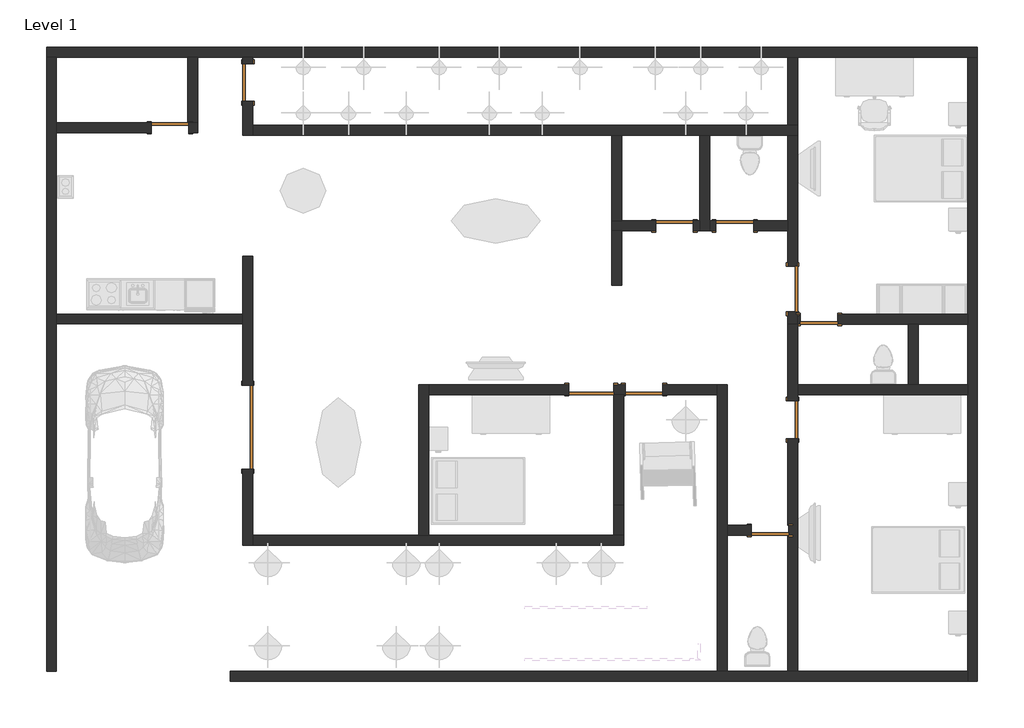
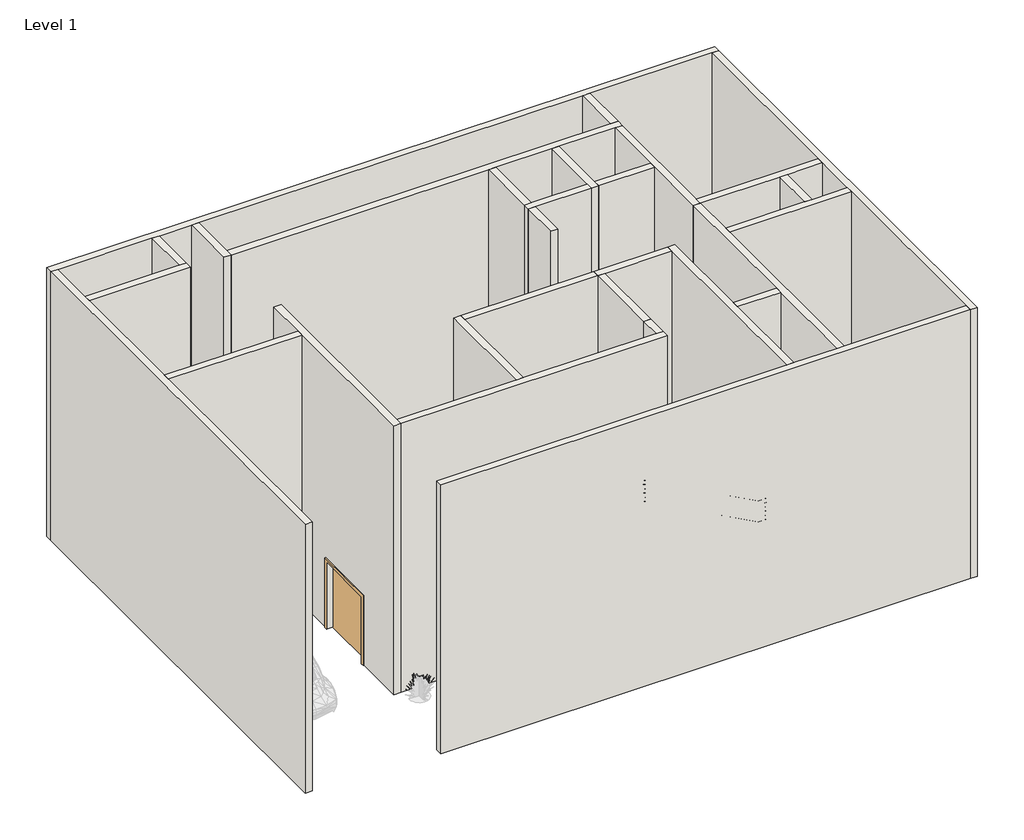
# One storey, part 1 of 4: 29 walls, 11 doors.
"""IFC4 building model written with IfcOpenShell, lengths in millimetres."""

from ifc_helpers import new_model, si_unit, frame, origin, origin_with_axes, place, context, project, spatial, polyline, outline, extrude, faceted_brep, transform, mapped, element, save
from components import m_door_double_flush_panel_double_acting_1700_x_2000mm_0a6d9c7f, m_single_flush_0762_x_2032mm_0c256fab, m_single_flush_0762_x_2032mm_7341a4fb, m_single_flush_0915_x_2032mm_26613924, m_single_flush_0915_x_2134mm_6a9e8738

model = new_model("IFC4")

# Units and contexts
model_context = context("Model", 3, world=origin())
ifc_project = project(units=[si_unit("LENGTHUNIT", "METRE", prefix="MILLI")], contexts=[model_context])

# Site, building, storey
site = spatial("IfcSite", under=ifc_project)
building = spatial("IfcBuilding", under=site)
storey = spatial("IfcBuildingStorey", under=building, Name="Level 1", Elevation=0.0)

# Doors
placement = place(None, origin())
m_door_double_flush_panel_double_acting_1700_x_2000mm_shape = m_door_double_flush_panel_double_acting_1700_x_2000mm_0a6d9c7f(model_context)
element("IfcDoor", 1, ObjectType="M_Door-Double-Flush_Panel-Double-Acting : 1700 x 2000mm", at=placement, inside=storey, context=model_context, shape_type="MappedRepresentation", body=[
    mapped(m_door_double_flush_panel_double_acting_1700_x_2000mm_shape, transform((-5650.4268643, 2289.4971112, 0.0), x_axis=(0.0, -1.0, 0.0), y_axis=(1.0, 0.0, 0.0), z_axis=(0.0, 0.0, 1.0))),
])
m_single_flush_0762_x_2032mm_shape = m_single_flush_0762_x_2032mm_0c256fab(model_context)
element("IfcDoor", 2, ObjectType="M_Single-Flush : 0762 x 2032mm", at=placement, inside=storey, context=model_context, shape_type="MappedRepresentation", body=[
    mapped(m_single_flush_0762_x_2032mm_shape, transform((-7222.0268643, 8333.0971112, 0.0), x_axis=(1.0, 0.0, 0.0), y_axis=(0.0, 1.0, 0.0), z_axis=(0.0, 0.0, 1.0))),
])
element("IfcDoor", 3, ObjectType="M_Single-Flush : 0762 x 2032mm", at=placement, inside=storey, context=model_context, shape_type="MappedRepresentation", body=[
    mapped(m_single_flush_0762_x_2032mm_shape, transform((-5648.8268643, 9249.0971112, 0.0), x_axis=(0.0, 1.0, 0.0), y_axis=(-1.0, 0.0, 0.0), z_axis=(0.0, 0.0, 1.0))),
])
element("IfcDoor", 4, ObjectType="M_Single-Flush : 0762 x 2032mm", at=placement, inside=storey, context=model_context, shape_type="MappedRepresentation", body=[
    mapped(m_single_flush_0762_x_2032mm_shape, transform((2963.3731357, 6351.8971112, 0.0), x_axis=(1.0, 0.0, 0.0), y_axis=(0.0, 1.0, 0.0), z_axis=(0.0, 0.0, 1.0))),
])
element("IfcDoor", 5, ObjectType="M_Single-Flush : 0762 x 2032mm", at=placement, inside=storey, context=model_context, shape_type="MappedRepresentation", body=[
    mapped(m_single_flush_0762_x_2032mm_shape, transform((5882.7731357, 4465.8971112, 0.0), x_axis=(-1.0, 0.0, 0.0), y_axis=(0.0, -1.0, 0.0), z_axis=(0.0, 0.0, 1.0))),
])
element("IfcDoor", 6, ObjectType="M_Single-Flush : 0762 x 2032mm", at=placement, inside=storey, context=model_context, shape_type="MappedRepresentation", body=[
    mapped(m_single_flush_0762_x_2032mm_shape, transform((2350.5731357, 3046.6971112, 0.0), x_axis=(-1.0, 0.0, 0.0), y_axis=(0.0, -1.0, 0.0), z_axis=(0.0, 0.0, 1.0))),
])
m_single_flush_0762_x_2032mm_2_shape = m_single_flush_0762_x_2032mm_7341a4fb(model_context)
element("IfcDoor", 7, ObjectType="M_Single-Flush : 0762 x 2032mm", at=placement, inside=storey, context=model_context, shape_type="MappedRepresentation", body=[
    mapped(m_single_flush_0762_x_2032mm_2_shape, transform((4182.5731357, 6351.8971112, 0.0), x_axis=(-1.0, 0.0, 0.0), y_axis=(0.0, -1.0, 0.0), z_axis=(0.0, 0.0, 1.0))),
])
element("IfcDoor", 8, ObjectType="M_Single-Flush : 0762 x 2032mm", at=placement, inside=storey, context=model_context, shape_type="MappedRepresentation", body=[
    mapped(m_single_flush_0762_x_2032mm_2_shape, transform((5349.3731357, 2437.0971112, 0.0), x_axis=(0.0, 1.0, 0.0), y_axis=(-1.0, 0.0, 0.0), z_axis=(0.0, 0.0, 1.0))),
])
element("IfcDoor", 9, ObjectType="M_Single-Flush : 0762 x 2032mm", at=placement, inside=storey, context=model_context, shape_type="MappedRepresentation", body=[
    mapped(m_single_flush_0762_x_2032mm_2_shape, transform((4892.1731357, 206.6971112, 0.0), x_axis=(1.0, 0.0, 0.0), y_axis=(0.0, 1.0, 0.0), z_axis=(0.0, 0.0, 1.0))),
])
m_single_flush_0915_x_2032mm_shape = m_single_flush_0915_x_2032mm_26613924(model_context)
element("IfcDoor", 10, ObjectType="M_Single-Flush : 0915 x 2032mm", at=placement, inside=storey, context=model_context, shape_type="MappedRepresentation", body=[
    mapped(m_single_flush_0915_x_2032mm_shape, transform((1283.7731357, 3046.6971112, 0.0), x_axis=(1.0, 0.0, 0.0), y_axis=(0.0, 1.0, 0.0), z_axis=(0.0, 0.0, 1.0))),
])
m_single_flush_0915_x_2134mm_shape = m_single_flush_0915_x_2134mm_6a9e8738(model_context)
element("IfcDoor", 11, ObjectType="M_Single-Flush : 0915 x 2134mm", at=placement, inside=storey, context=model_context, shape_type="MappedRepresentation", body=[
    mapped(m_single_flush_0915_x_2134mm_shape, transform((5349.3731357, 5075.4971112, 0.0), x_axis=(0.0, -1.0, 0.0), y_axis=(1.0, 0.0, 0.0), z_axis=(0.0, 0.0, 1.0))),
])

# Walls
element("IfcWall", 12, ObjectType="Generic - 200mm", at=placement, inside=storey, context=model_context, shape_type="Brep", body=[
    faceted_brep([(-9712.8268643, 9758.6971112, 0.0), (-9512.8268643, 9758.6971112, 0.0), (-6864.8268643, 9758.6971112, 0.0), (-6664.8268643, 9758.6971112, 0.0), (-5748.8268643, 9758.6971112, 0.0), (-5548.8268643, 9758.6971112, 0.0), (5249.3731357, 9758.6971112, 0.0), (5449.3731357, 9758.6971112, 0.0), (8879.9731357, 9758.6971112, 0.0), (9079.9731357, 9758.6971112, 0.0), (9079.9731357, 9758.6971112, 8000.0), (8879.9731357, 9758.6971112, 8000.0), (5449.3731357, 9758.6971112, 8000.0), (5249.3731357, 9758.6971112, 8000.0), (-5548.8268643, 9758.6971112, 8000.0), (-5748.8268643, 9758.6971112, 8000.0), (-6664.8268643, 9758.6971112, 8000.0), (-6864.8268643, 9758.6971112, 8000.0), (-9512.8268643, 9758.6971112, 8000.0), (-9712.8268643, 9758.6971112, 8000.0), (-9712.8268643, 9958.6971112, 0.0), (-9712.8268643, 9958.6971112, 8000.0), (9079.9731357, 9958.6971112, 8000.0), (9079.9731357, 9958.6971112, 0.0)], [[[0, 1, 2, 3, 4, 5, 6, 7, 8, 9, 10, 11, 12, 13, 14, 15, 16, 17, 18, 19]], [[20, 21, 22, 23]], [[9, 8, 7, 6, 5, 4, 3, 2, 1, 0, 20, 23]], [[19, 18, 17, 16, 15, 14, 13, 12, 11, 10, 22, 21]], [[10, 9, 23, 22]], [[0, 19, 21, 20]]]),
])
element("IfcWall", 13, ObjectType="Generic - 200mm", at=placement, inside=storey, context=model_context, shape_type="Brep", body=[
    faceted_brep([(8879.9731357, 9758.6971112, 0.0), (8879.9731357, 4565.8971112, 0.0), (8879.9731357, 4365.8971112, 0.0), (8879.9731357, 3146.6971112, 0.0), (8879.9731357, 2946.6971112, 0.0), (8879.9731357, -2638.1028888, 0.0), (8879.9731357, -2838.1028888, 0.0), (8879.9731357, -2838.1028888, 8000.0), (8879.9731357, -2638.1028888, 8000.0), (8879.9731357, 2946.6971112, 8000.0), (8879.9731357, 3146.6971112, 8000.0), (8879.9731357, 4365.8971112, 8000.0), (8879.9731357, 4565.8971112, 8000.0), (8879.9731357, 9758.6971112, 8000.0), (9079.9731357, 9758.6971112, 0.0), (9079.9731357, 9758.6971112, 8000.0), (9079.9731357, -2838.1028888, 8000.0), (9079.9731357, -2838.1028888, 0.0)], [[[0, 1, 2, 3, 4, 5, 6, 7, 8, 9, 10, 11, 12, 13]], [[14, 15, 16, 17]], [[6, 5, 4, 3, 2, 1, 0, 14, 17]], [[13, 12, 11, 10, 9, 8, 7, 16, 15]], [[0, 13, 15, 14]], [[7, 6, 17, 16]]]),
])
element("IfcWall", 14, ObjectType="Generic - 200mm", at=placement, inside=storey, context=model_context, shape_type="Brep", body=[
    faceted_brep([(-9512.8268643, -2638.1028888, 0.0), (-9512.8268643, 4372.2971112, 0.0), (-9512.8268643, 4572.2971112, 0.0), (-9512.8268643, 8233.0971112, 0.0), (-9512.8268643, 8433.0971112, 0.0), (-9512.8268643, 9758.6971112, 0.0), (-9512.8268643, 9758.6971112, 8000.0), (-9512.8268643, 8433.0971112, 8000.0), (-9512.8268643, 8233.0971112, 8000.0), (-9512.8268643, 4572.2971112, 8000.0), (-9512.8268643, 4372.2971112, 8000.0), (-9512.8268643, -2638.1028888, 8000.0), (-9712.8268643, -2638.1028888, 0.0), (-9712.8268643, -2638.1028888, 8000.0), (-9712.8268643, 9758.6971112, 8000.0), (-9712.8268643, 9758.6971112, 0.0)], [[[0, 1, 2, 3, 4, 5, 6, 7, 8, 9, 10, 11]], [[12, 13, 14, 15]], [[5, 4, 3, 2, 1, 0, 12, 15]], [[11, 10, 9, 8, 7, 6, 14, 13]], [[0, 11, 13, 12]], [[6, 5, 15, 14]]]),
])
element("IfcWall", 15, ObjectType="Generic - 200mm", at=placement, inside=storey, context=model_context, shape_type="Brep", body=[
    faceted_brep([(-6841.0268643, 8233.0971112, 2032.0), (-6841.0268643, 8233.0971112, 0.0), (-6664.8268643, 8233.0971112, 0.0), (-6664.8268643, 8233.0971112, 8000.0), (-9512.8268643, 8233.0971112, 8000.0), (-9512.8268643, 8233.0971112, 0.0), (-7603.0268643, 8233.0971112, 0.0), (-7603.0268643, 8233.0971112, 2032.0), (-6664.8268643, 8433.0971112, 0.0), (-6841.0268643, 8433.0971112, 0.0), (-6841.0268643, 8433.0971112, 2032.0), (-7603.0268643, 8433.0971112, 2032.0), (-7603.0268643, 8433.0971112, 0.0), (-9512.8268643, 8433.0971112, 0.0), (-9512.8268643, 8433.0971112, 8000.0), (-6864.8268643, 8433.0971112, 8000.0), (-6664.8268643, 8433.0971112, 8000.0)], [[[0, 1, 2, 3, 4, 5, 6, 7]], [[8, 9, 10, 11, 12, 13, 14, 15, 16]], [[6, 5, 13, 12]], [[2, 1, 9, 8]], [[4, 3, 16, 15, 14]], [[5, 4, 14, 13]], [[3, 2, 8, 16]], [[10, 9, 1, 0]], [[11, 10, 0, 7]], [[12, 11, 7, 6]]]),
])
element("IfcWall", 16, ObjectType="Generic - 200mm", at=placement, inside=storey, context=model_context, shape_type="SweptSolid", body=[
    extrude(outline(polyline([(-6664.8268643, 9758.6971112), (-6664.8268643, 8433.0971112), (-6864.8268643, 8433.0971112), (-6864.8268643, 9758.6971112), (-6664.8268643, 9758.6971112)])), origin_with_axes(), (0.0, 0.0, 1.0), 8000.0),
])
element("IfcWall", 17, ObjectType="Generic - 200mm", at=placement, inside=storey, context=model_context, shape_type="SweptSolid", body=[
    extrude(outline(polyline([(-5750.4268643, 4372.2971112), (-9512.8268643, 4372.2971112), (-9512.8268643, 4572.2971112), (-5750.4268643, 4572.2971112), (-5750.4268643, 4372.2971112)])), origin_with_axes(), (0.0, 0.0, 1.0), 8000.0),
])
element("IfcWall", 18, ObjectType="Generic - 200mm", at=placement, inside=storey, context=model_context, shape_type="Brep", body=[
    faceted_brep([(-5550.4268643, 5743.8971112, 0.0), (-5550.4268643, 5743.8971112, 8000.0), (-5550.4268643, 106.6971112, 8000.0), (-5550.4268643, -93.3028888, 8000.0), (-5550.4268643, -93.3028888, 0.0), (-5550.4268643, 106.6971112, 0.0), (-5550.4268643, 1439.4971112, 0.0), (-5550.4268643, 1439.4971112, 2000.0), (-5550.4268643, 3139.4971112, 2000.0), (-5550.4268643, 3139.4971112, 0.0), (-5750.4268643, 5743.8971112, 8000.0), (-5750.4268643, 5743.8971112, 0.0), (-5750.4268643, 4572.2971112, 0.0), (-5750.4268643, 4372.2971112, 0.0), (-5750.4268643, 3139.4971112, 0.0), (-5750.4268643, 3139.4971112, 2000.0), (-5750.4268643, 1439.4971112, 2000.0), (-5750.4268643, 1439.4971112, 0.0), (-5750.4268643, -93.3028888, 0.0), (-5750.4268643, -93.3028888, 8000.0), (-5750.4268643, 4372.2971112, 8000.0), (-5750.4268643, 4572.2971112, 8000.0)], [[[0, 1, 2, 3, 4, 5, 6, 7, 8, 9]], [[10, 11, 12, 13, 14, 15, 16, 17, 18, 19, 20, 21]], [[11, 0, 9, 14, 13, 12]], [[4, 18, 17, 6, 5]], [[1, 0, 11, 10]], [[3, 2, 1, 10, 21, 20, 19]], [[16, 7, 6, 17]], [[7, 16, 15, 8]], [[8, 15, 14, 9]], [[4, 3, 19, 18]]]),
])
element("IfcWall", 19, ObjectType="Generic - 200mm", at=placement, inside=storey, context=model_context, shape_type="Brep", body=[
    faceted_brep([(-5748.8268643, 9758.6971112, 0.0), (-5748.8268643, 9630.0971112, 0.0), (-5748.8268643, 9630.0971112, 2032.0), (-5748.8268643, 8868.0971112, 2032.0), (-5748.8268643, 8868.0971112, 0.0), (-5748.8268643, 8180.6971112, 0.0), (-5748.8268643, 8180.6971112, 8000.0), (-5748.8268643, 9758.6971112, 8000.0), (-5548.8268643, 9630.0971112, 2032.0), (-5548.8268643, 9630.0971112, 0.0), (-5548.8268643, 9758.6971112, 0.0), (-5548.8268643, 9758.6971112, 8000.0), (-5548.8268643, 8380.6971112, 8000.0), (-5548.8268643, 8180.6971112, 8000.0), (-5548.8268643, 8180.6971112, 0.0), (-5548.8268643, 8380.6971112, 0.0), (-5548.8268643, 8868.0971112, 0.0), (-5548.8268643, 8868.0971112, 2032.0)], [[[0, 1, 2, 3, 4, 5, 6, 7]], [[8, 9, 10, 11, 12, 13, 14, 15, 16, 17]], [[10, 9, 1, 0]], [[16, 15, 14, 5, 4]], [[6, 5, 14, 13]], [[7, 6, 13, 12, 11]], [[0, 7, 11, 10]], [[2, 1, 9, 8]], [[3, 2, 8, 17]], [[4, 3, 17, 16]]]),
])
element("IfcWall", 20, ObjectType="Generic - 200mm", at=placement, inside=storey, context=model_context, shape_type="Brep", body=[
    faceted_brep([(-5548.8268643, 8180.6971112, 0.0), (1694.9731357, 8180.6971112, 0.0), (1894.9731357, 8180.6971112, 0.0), (3472.9731357, 8180.6971112, 0.0), (3672.9731357, 8180.6971112, 0.0), (5249.3731357, 8180.6971112, 0.0), (5449.3731357, 8180.6971112, 0.0), (5449.3731357, 8180.6971112, 8000.0), (5249.3731357, 8180.6971112, 8000.0), (3672.9731357, 8180.6971112, 8000.0), (3472.9731357, 8180.6971112, 8000.0), (1894.9731357, 8180.6971112, 8000.0), (1694.9731357, 8180.6971112, 8000.0), (-5548.8268643, 8180.6971112, 8000.0), (-5548.8268643, 8380.6971112, 0.0), (-5548.8268643, 8380.6971112, 8000.0), (5249.3731357, 8380.6971112, 8000.0), (5449.3731357, 8380.6971112, 8000.0), (5449.3731357, 8380.6971112, 0.0), (5249.3731357, 8380.6971112, 0.0)], [[[0, 1, 2, 3, 4, 5, 6, 7, 8, 9, 10, 11, 12, 13]], [[14, 15, 16, 17, 18, 19]], [[6, 5, 4, 3, 2, 1, 0, 14, 19, 18]], [[13, 12, 11, 10, 9, 8, 7, 17, 16, 15]], [[0, 13, 15, 14]], [[7, 6, 18, 17]]]),
])
element("IfcWall", 21, ObjectType="Generic - 200mm", at=placement, inside=storey, context=model_context, shape_type="SweptSolid", body=[
    extrude(outline(polyline([(5449.3731357, 9758.6971112), (5449.3731357, 8380.6971112), (5249.3731357, 8380.6971112), (5249.3731357, 9758.6971112), (5449.3731357, 9758.6971112)])), origin_with_axes(), (0.0, 0.0, 1.0), 8000.0),
])
element("IfcWall", 22, ObjectType="Generic - 200mm", at=placement, inside=storey, context=model_context, shape_type="Brep", body=[
    faceted_brep([(5249.3731357, 4617.9971112, 2134.0), (5249.3731357, 4617.9971112, 0.0), (5249.3731357, 4365.8971112, 0.0), (5249.3731357, 4365.8971112, 8000.0), (5249.3731357, 6251.8971112, 8000.0), (5249.3731357, 6451.8971112, 8000.0), (5249.3731357, 8180.6971112, 8000.0), (5249.3731357, 8180.6971112, 0.0), (5249.3731357, 6451.8971112, 0.0), (5249.3731357, 6251.8971112, 0.0), (5249.3731357, 5532.9971112, 0.0), (5249.3731357, 5532.9971112, 2134.0), (5449.3731357, 4365.8971112, 0.0), (5449.3731357, 4565.8971112, 0.0), (5449.3731357, 4617.9971112, 0.0), (5449.3731357, 4617.9971112, 2134.0), (5449.3731357, 5532.9971112, 2134.0), (5449.3731357, 5532.9971112, 0.0), (5449.3731357, 8180.6971112, 0.0), (5449.3731357, 8180.6971112, 8000.0), (5449.3731357, 4565.8971112, 8000.0), (5449.3731357, 4365.8971112, 8000.0)], [[[0, 1, 2, 3, 4, 5, 6, 7, 8, 9, 10, 11]], [[12, 13, 14, 15, 16, 17, 18, 19, 20, 21]], [[2, 1, 14, 13, 12]], [[10, 9, 8, 7, 18, 17]], [[6, 5, 4, 3, 21, 20, 19]], [[7, 6, 19, 18]], [[3, 2, 12, 21]], [[15, 14, 1, 0]], [[16, 15, 0, 11]], [[17, 16, 11, 10]]]),
])
element("IfcWall", 23, ObjectType="Generic - 200mm", at=placement, inside=storey, context=model_context, shape_type="Brep", body=[
    faceted_brep([(5449.3731357, 4365.8971112, 0.0), (5501.7731357, 4365.8971112, 0.0), (5501.7731357, 4365.8971112, 2032.0), (6263.7731357, 4365.8971112, 2032.0), (6263.7731357, 4365.8971112, 0.0), (7684.5731357, 4365.8971112, 0.0), (7884.5731357, 4365.8971112, 0.0), (8879.9731357, 4365.8971112, 0.0), (8879.9731357, 4365.8971112, 8000.0), (7884.5731357, 4365.8971112, 8000.0), (7684.5731357, 4365.8971112, 8000.0), (5449.3731357, 4365.8971112, 8000.0), (5501.7731357, 4565.8971112, 2032.0), (5501.7731357, 4565.8971112, 0.0), (5449.3731357, 4565.8971112, 0.0), (5449.3731357, 4565.8971112, 8000.0), (8879.9731357, 4565.8971112, 8000.0), (8879.9731357, 4565.8971112, 0.0), (6263.7731357, 4565.8971112, 0.0), (6263.7731357, 4565.8971112, 2032.0)], [[[0, 1, 2, 3, 4, 5, 6, 7, 8, 9, 10, 11]], [[12, 13, 14, 15, 16, 17, 18, 19]], [[18, 17, 7, 6, 5, 4]], [[14, 13, 1, 0]], [[11, 10, 9, 8, 16, 15]], [[0, 11, 15, 14]], [[8, 7, 17, 16]], [[2, 1, 13, 12]], [[3, 2, 12, 19]], [[4, 3, 19, 18]]]),
])
element("IfcWall", 24, ObjectType="Generic - 200mm", at=placement, inside=storey, context=model_context, shape_type="Brep", body=[
    faceted_brep([(3472.9731357, 8180.6971112, 0.0), (3472.9731357, 6451.8971112, 0.0), (3472.9731357, 6251.8971112, 0.0), (3472.9731357, 6251.8971112, 8000.0), (3472.9731357, 6451.8971112, 8000.0), (3472.9731357, 8180.6971112, 8000.0), (3672.9731357, 8180.6971112, 0.0), (3672.9731357, 8180.6971112, 8000.0), (3672.9731357, 6451.8971112, 8000.0), (3672.9731357, 6251.8971112, 8000.0), (3672.9731357, 6251.8971112, 0.0), (3672.9731357, 6451.8971112, 0.0)], [[[0, 1, 2, 3, 4, 5]], [[6, 7, 8, 9, 10, 11]], [[2, 1, 0, 6, 11, 10]], [[5, 4, 3, 9, 8, 7]], [[0, 5, 7, 6]], [[3, 2, 10, 9]]]),
])
element("IfcWall", 25, ObjectType="Generic - 200mm", at=placement, inside=storey, context=model_context, shape_type="SweptSolid", body=[
    extrude(outline(polyline([(0.0, 3672.9731357), (0.0, 3801.5731357), (2032.0, 3801.5731357), (2032.0, 4563.5731357), (0.0, 4563.5731357), (0.0, 5249.3731357), (8000.0, 5249.3731357), (8000.0, 3672.9731357), (0.0, 3672.9731357)])), frame((0.0, 6251.8971112, 0.0), z_axis=(0.0, 1.0, 0.0), x_axis=(0.0, 0.0, 1.0)), (0.0, 0.0, 1.0), 200.0),
])
element("IfcWall", 26, ObjectType="Generic - 200mm", at=placement, inside=storey, context=model_context, shape_type="Brep", body=[
    faceted_brep([(3472.9731357, 6451.8971112, 0.0), (3344.3731357, 6451.8971112, 0.0), (3344.3731357, 6451.8971112, 2032.0), (2582.3731357, 6451.8971112, 2032.0), (2582.3731357, 6451.8971112, 0.0), (1894.9731357, 6451.8971112, 0.0), (1694.9731357, 6451.8971112, 0.0), (1694.9731357, 6451.8971112, 8000.0), (1894.9731357, 6451.8971112, 8000.0), (3472.9731357, 6451.8971112, 8000.0), (3344.3731357, 6251.8971112, 2032.0), (3344.3731357, 6251.8971112, 0.0), (3472.9731357, 6251.8971112, 0.0), (3472.9731357, 6251.8971112, 8000.0), (1896.5731357, 6251.8971112, 8000.0), (1696.5731357, 6251.8971112, 8000.0), (1694.9731357, 6251.8971112, 8000.0), (1694.9731357, 6251.8971112, 0.0), (1696.5731357, 6251.8971112, 0.0), (1896.5731357, 6251.8971112, 0.0), (2582.3731357, 6251.8971112, 0.0), (2582.3731357, 6251.8971112, 2032.0)], [[[0, 1, 2, 3, 4, 5, 6, 7, 8, 9]], [[10, 11, 12, 13, 14, 15, 16, 17, 18, 19, 20, 21]], [[12, 11, 1, 0]], [[20, 19, 18, 17, 6, 5, 4]], [[9, 8, 7, 16, 15, 14, 13]], [[0, 9, 13, 12]], [[7, 6, 17, 16]], [[2, 1, 11, 10]], [[3, 2, 10, 21]], [[4, 3, 21, 20]]]),
])
element("IfcWall", 27, ObjectType="Generic - 200mm", at=placement, inside=storey, context=model_context, shape_type="SweptSolid", body=[
    extrude(outline(polyline([(1894.9731357, 8180.6971112), (1894.9731357, 6451.8971112), (1694.9731357, 6451.8971112), (1694.9731357, 8180.6971112), (1894.9731357, 8180.6971112)])), origin_with_axes(), (0.0, 0.0, 1.0), 8000.0),
])
element("IfcWall", 28, ObjectType="Generic - 200mm", at=placement, inside=storey, context=model_context, shape_type="Brep", body=[
    faceted_brep([(5249.3731357, -2638.1028888, 8000.0), (5249.3731357, 106.6971112, 8000.0), (5249.3731357, 306.6971112, 8000.0), (5249.3731357, 4365.8971112, 8000.0), (5249.3731357, 4365.8971112, 0.0), (5249.3731357, 2818.0971112, 0.0), (5249.3731357, 2818.0971112, 2032.0), (5249.3731357, 2056.0971112, 2032.0), (5249.3731357, 2056.0971112, 0.0), (5249.3731357, 306.6971112, 0.0), (5249.3731357, 306.6971112, 2032.0), (5249.3731357, 106.6971112, 2032.0), (5249.3731357, 106.6971112, 0.0), (5249.3731357, -2638.1028888, 0.0), (5449.3731357, 4365.8971112, 8000.0), (5449.3731357, 3146.6971112, 8000.0), (5449.3731357, 2946.6971112, 8000.0), (5449.3731357, -2638.1028888, 8000.0), (5449.3731357, -2638.1028888, 0.0), (5449.3731357, 2056.0971112, 0.0), (5449.3731357, 2056.0971112, 2032.0), (5449.3731357, 2818.0971112, 2032.0), (5449.3731357, 2818.0971112, 0.0), (5449.3731357, 2946.6971112, 0.0), (5449.3731357, 3146.6971112, 0.0), (5449.3731357, 4365.8971112, 0.0), (5273.1731357, 106.6971112, 0.0), (5273.1731357, 306.6971112, 0.0), (5273.1731357, 106.6971112, 2032.0), (5273.1731357, 306.6971112, 2032.0)], [[[0, 1, 2, 3, 4, 5, 6, 7, 8, 9, 10, 11, 12, 13]], [[14, 15, 16, 17, 18, 19, 20, 21, 22, 23, 24, 25]], [[4, 25, 24, 23, 22, 5]], [[8, 19, 18, 13, 12, 26, 27, 9]], [[3, 2, 1, 0, 17, 16, 15, 14]], [[4, 3, 14, 25]], [[6, 5, 22, 21]], [[7, 6, 21, 20]], [[8, 7, 20, 19]], [[28, 26, 12, 11]], [[27, 29, 10, 9]], [[26, 28, 29, 27]], [[29, 28, 11, 10]], [[0, 13, 18, 17]]]),
])
element("IfcWall", 29, ObjectType="Generic - 200mm", at=placement, inside=storey, context=model_context, shape_type="Brep", body=[
    faceted_brep([(5449.3731357, 2946.6971112, 0.0), (8879.9731357, 2946.6971112, 0.0), (8879.9731357, 2946.6971112, 8000.0), (5449.3731357, 2946.6971112, 8000.0), (5449.3731357, 3146.6971112, 0.0), (5449.3731357, 3146.6971112, 8000.0), (7684.5731357, 3146.6971112, 8000.0), (7884.5731357, 3146.6971112, 8000.0), (8879.9731357, 3146.6971112, 8000.0), (8879.9731357, 3146.6971112, 0.0), (7884.5731357, 3146.6971112, 0.0), (7684.5731357, 3146.6971112, 0.0)], [[[0, 1, 2, 3]], [[4, 5, 6, 7, 8, 9, 10, 11]], [[1, 0, 4, 11, 10, 9]], [[3, 2, 8, 7, 6, 5]], [[0, 3, 5, 4]], [[2, 1, 9, 8]]]),
])
element("IfcWall", 30, ObjectType="Generic - 200mm", at=placement, inside=storey, context=model_context, shape_type="SweptSolid", body=[
    extrude(outline(polyline([(7884.5731357, 4365.8971112), (7884.5731357, 3146.6971112), (7684.5731357, 3146.6971112), (7684.5731357, 4365.8971112), (7884.5731357, 4365.8971112)])), origin_with_axes(), (0.0, 0.0, 1.0), 8000.0),
])
element("IfcWall", 31, ObjectType="Generic - 200mm", at=placement, inside=storey, context=model_context, shape_type="SweptSolid", body=[
    extrude(outline(polyline([(1696.5731357, 5158.0971112), (1696.5731357, 6251.8971112), (1896.5731357, 6251.8971112), (1896.5731357, 5158.0971112), (1696.5731357, 5158.0971112)])), origin_with_axes(), (0.0, 0.0, 1.0), 8000.0),
])
element("IfcWall", 32, ObjectType="Generic - 200mm", at=placement, inside=storey, context=model_context, shape_type="Brep", body=[
    faceted_brep([(4026.9731357, -2638.1028888, 0.0), (4026.9731357, 106.6971112, 0.0), (4026.9731357, 306.6971112, 0.0), (4026.9731357, 3146.6971112, 0.0), (4026.9731357, 3146.6971112, 8000.0), (4026.9731357, 306.6971112, 8000.0), (4026.9731357, 106.6971112, 8000.0), (4026.9731357, -2638.1028888, 8000.0), (3826.9731357, -2638.1028888, 0.0), (3826.9731357, -2638.1028888, 8000.0), (3826.9731357, 2946.6971112, 8000.0), (3826.9731357, 3146.6971112, 8000.0), (3826.9731357, 3146.6971112, 0.0), (3826.9731357, 2946.6971112, 0.0)], [[[0, 1, 2, 3, 4, 5, 6, 7]], [[8, 9, 10, 11, 12, 13]], [[3, 2, 1, 0, 8, 13, 12]], [[7, 6, 5, 4, 11, 10, 9]], [[4, 3, 12, 11]], [[0, 7, 9, 8]]]),
])
element("IfcWall", 33, ObjectType="Generic - 200mm", at=placement, inside=storey, context=model_context, shape_type="SweptSolid", body=[
    extrude(outline(polyline([(8000.0, 5249.3731357), (8000.0, 4026.9731357), (0.0, 4026.9731357), (0.0, 4511.1731357), (2032.0, 4511.1731357), (2032.0, 5249.3731357), (8000.0, 5249.3731357)])), frame((0.0, 106.6971112, 0.0), z_axis=(0.0, 1.0, 0.0), x_axis=(0.0, 0.0, 1.0)), (0.0, 0.0, 1.0), 200.0),
])
element("IfcWall", 34, ObjectType="Generic - 200mm", at=placement, inside=storey, context=model_context, shape_type="Brep", body=[
    faceted_brep([(1969.5731357, 3146.6971112, 2032.0), (1969.5731357, 3146.6971112, 0.0), (1741.2731357, 3146.6971112, 0.0), (1741.2731357, 3146.6971112, 2032.0), (1740.9731357, 3146.6971112, 2032.0), (1740.9731357, 3146.6971112, 8000.0), (3826.9731357, 3146.6971112, 8000.0), (3826.9731357, 3146.6971112, 0.0), (2731.5731357, 3146.6971112, 0.0), (2731.5731357, 3146.6971112, 2032.0), (1741.2731357, 2946.6971112, 0.0), (1940.9731357, 2946.6971112, 0.0), (1969.5731357, 2946.6971112, 0.0), (1969.5731357, 2946.6971112, 2032.0), (2731.5731357, 2946.6971112, 2032.0), (2731.5731357, 2946.6971112, 0.0), (3826.9731357, 2946.6971112, 0.0), (3826.9731357, 2946.6971112, 8000.0), (1940.9731357, 2946.6971112, 8000.0), (1740.9731357, 2946.6971112, 8000.0), (1740.9731357, 2946.6971112, 2032.0), (1741.2731357, 2946.6971112, 2032.0)], [[[0, 1, 2, 3, 4, 5, 6, 7, 8, 9]], [[10, 11, 12, 13, 14, 15, 16, 17, 18, 19, 20, 21]], [[8, 7, 16, 15]], [[2, 1, 12, 11, 10]], [[6, 5, 19, 18, 17]], [[7, 6, 17, 16]], [[19, 5, 4, 20]], [[21, 3, 2, 10]], [[3, 21, 20, 4]], [[13, 12, 1, 0]], [[14, 13, 0, 9]], [[15, 14, 9, 8]]]),
])
element("IfcWall", 35, ObjectType="Generic - 200mm", at=placement, inside=storey, context=model_context, shape_type="Brep", body=[
    faceted_brep([(1740.9731357, 2946.6971112, 0.0), (1740.9731357, 708.2971112, 0.0), (1740.9731357, 708.2971112, 8000.0), (1740.9731357, 2946.6971112, 8000.0), (1740.9731357, 2946.6971112, 2032.0), (1940.9731357, 2946.6971112, 0.0), (1940.9731357, 2946.6971112, 8000.0), (1940.9731357, 708.2971112, 8000.0), (1940.9731357, 708.2971112, 0.0), (1741.2731357, 2946.6971112, 0.0)], [[[0, 1, 2, 3, 4]], [[5, 6, 7, 8]], [[1, 0, 9, 5, 8]], [[2, 1, 8, 7]], [[3, 2, 7, 6]], [[0, 4, 3, 6, 5, 9]]]),
])
element("IfcWall", 36, ObjectType="Generic - 200mm", at=placement, inside=storey, context=model_context, shape_type="Brep", body=[
    faceted_brep([(-5550.4268643, -93.3028888, 0.0), (1940.9731357, -93.3028888, 0.0), (1940.9731357, -93.3028888, 8000.0), (-5550.4268643, -93.3028888, 8000.0), (-5550.4268643, 106.6971112, 0.0), (-5550.4268643, 106.6971112, 8000.0), (-2194.4268643, 106.6971112, 8000.0), (-1994.4268643, 106.6971112, 8000.0), (1740.9731357, 106.6971112, 8000.0), (1940.9731357, 106.6971112, 8000.0), (1940.9731357, 106.6971112, 0.0), (1740.9731357, 106.6971112, 0.0), (-1994.4268643, 106.6971112, 0.0), (-2194.4268643, 106.6971112, 0.0)], [[[0, 1, 2, 3]], [[4, 5, 6, 7, 8, 9, 10, 11, 12, 13]], [[1, 0, 4, 13, 12, 11, 10]], [[3, 2, 9, 8, 7, 6, 5]], [[0, 3, 5, 4]], [[2, 1, 10, 9]]]),
])
element("IfcWall", 37, ObjectType="Generic - 200mm", at=placement, inside=storey, context=model_context, shape_type="Brep", body=[
    faceted_brep([(-1994.4268643, 106.6971112, 0.0), (-1994.4268643, 2946.6971112, 0.0), (-1994.4268643, 3146.6971112, 0.0), (-1994.4268643, 3146.6971112, 8000.0), (-1994.4268643, 2946.6971112, 8000.0), (-1994.4268643, 106.6971112, 8000.0), (-2194.4268643, 106.6971112, 0.0), (-2194.4268643, 106.6971112, 8000.0), (-2194.4268643, 3146.6971112, 8000.0), (-2194.4268643, 3146.6971112, 0.0)], [[[0, 1, 2, 3, 4, 5]], [[6, 7, 8, 9]], [[2, 1, 0, 6, 9]], [[5, 4, 3, 8, 7]], [[0, 5, 7, 6]], [[3, 2, 9, 8]]]),
])
element("IfcWall", 38, ObjectType="Generic - 200mm", at=placement, inside=storey, context=model_context, shape_type="SweptSolid", body=[
    extrude(outline(polyline([(8000.0, 1740.9731357), (8000.0, -1994.4268643), (0.0, -1994.4268643), (0.0, 826.2731357), (2032.0, 826.2731357), (2032.0, 1740.9731357), (8000.0, 1740.9731357)])), frame((0.0, 2946.6971112, 0.0), z_axis=(0.0, 1.0, 0.0), x_axis=(0.0, 0.0, 1.0)), (0.0, 0.0, 1.0), 200.0),
])
element("IfcWall", 39, ObjectType="Generic - 200mm", at=placement, inside=storey, context=model_context, shape_type="SweptSolid", body=[
    extrude(outline(polyline([(1940.9731357, 708.2971112), (1940.9731357, 106.6971112), (1740.9731357, 106.6971112), (1740.9731357, 708.2971112), (1940.9731357, 708.2971112)])), origin_with_axes(), (0.0, 0.0, 1.0), 8000.0),
])
element("IfcWall", 40, ObjectType="Generic - 200mm", at=placement, inside=storey, context=model_context, shape_type="Brep", body=[
    faceted_brep([(8879.9731357, -2638.1028888, 0.0), (5449.3731357, -2638.1028888, 0.0), (5249.3731357, -2638.1028888, 0.0), (4026.9731357, -2638.1028888, 0.0), (3826.9731357, -2638.1028888, 0.0), (-6007.6268643, -2638.1028888, 0.0), (-6007.6268643, -2638.1028888, 8000.0), (3826.9731357, -2638.1028888, 8000.0), (4026.9731357, -2638.1028888, 8000.0), (5249.3731357, -2638.1028888, 8000.0), (5449.3731357, -2638.1028888, 8000.0), (8879.9731357, -2638.1028888, 8000.0), (8879.9731357, -2838.1028888, 0.0), (8879.9731357, -2838.1028888, 8000.0), (-6007.6268643, -2838.1028888, 8000.0), (-6007.6268643, -2838.1028888, 0.0)], [[[0, 1, 2, 3, 4, 5, 6, 7, 8, 9, 10, 11]], [[12, 13, 14, 15]], [[5, 4, 3, 2, 1, 0, 12, 15]], [[6, 5, 15, 14]], [[11, 10, 9, 8, 7, 6, 14, 13]], [[0, 11, 13, 12]]]),
])

save(model, "model.ifc")

# Revit data of these elements
# Type "M_Door-Double-Flush_Panel-Double-Acting : 1700 x 2000mm"
#   Type Mark = "22"
#   Construction Type Id = "DOOR"
#   Assembly Code = "C1020"
#   Analytic Construction = "Wooden"
#   W = 850 mm
#   Thickness = 50 mm
#   Thermal Resistance (R) = 0.455703 (m²·K)/W
#   Swing Angle [instance default] = 90.00°
#   Heat Transfer Coefficient (U) = 2.19465 W/(m²·K)
#   Height = 2000 mm
#   Trim Projection Ext. = 25 mm
#   Trim Projection Int. = 25 mm
#   Trim Width Ext. = 80 mm
#   Trim Width Int. = 80 mm
#   Width = 1700 mm
#   Define Thermal Properties by = 1
#   Panel Material = Wood - Birch - Solid Stained Light Low Gloss
#   Trim Material = Paint - Sienna
#   Visual Light Transmittance = 0
#   Solar Heat Gain Coefficient = 0
#   Function = (empty or 0)
#   Wall Closure = (empty or 0)
# Type "M_Single-Flush : 0762 x 2032mm"
#   Type Mark = "19"
#   Thickness = 51 mm
#   Height = 2032 mm
#   Trim Projection Ext = 25 mm
#   Trim Projection Int = 25 mm
#   Trim Width = 76 mm
#   Width = 762 mm
#   Door Material = Door - Panel
#   Frame Material = Door - Frame
#   Function = (empty or 0)
#   Wall Closure = (empty or 0)
# Type "M_Single-Flush : 0915 x 2032mm"
#   Type Mark = "20"
#   Thickness = 51 mm
#   Height = 2032 mm
#   Trim Projection Ext = 25 mm
#   Trim Projection Int = 25 mm
#   Trim Width = 76 mm
#   Width = 915 mm
#   Door Material = Door - Panel
#   Frame Material = Door - Frame
#   Function = (empty or 0)
#   Wall Closure = (empty or 0)
# Type "M_Single-Flush : 0915 x 2134mm"
#   Type Mark = "15"
#   Thickness = 51 mm
#   Height = 2134 mm
#   Trim Projection Ext = 25 mm
#   Trim Projection Int = 25 mm
#   Trim Width = 76 mm
#   Width = 915 mm
#   Door Material = Door - Panel
#   Frame Material = Door - Frame
#   Function = (empty or 0)
#   Wall Closure = (empty or 0)
# Type "Generic - 200mm"
#   Layers, outside or top first: 200.025 mm no material (function 1)
# Element 1 (IfcDoor, "M_Door-Double-Flush_Panel-Double-Acting : 1700 x 2000mm")
#   Swing Angle = 90.00°
#   Phase Created = New Construction
#   Materials on its faces: "Paint - Sienna", "Wood - Birch - Solid Stained Light Low Gloss"
# Elements 2, 3, 4, 5, 6, 7, 8, 9 (IfcDoor, "M_Single-Flush : 0762 x 2032mm")
#   Phase Created = New Construction
#   Materials on its faces: "Door - Frame", "Door - Panel"
# Element 10 (IfcDoor, "M_Single-Flush : 0915 x 2032mm")
#   Phase Created = New Construction
#   Materials on its faces: "Door - Frame", "Door - Panel"
# Element 11 (IfcDoor, "M_Single-Flush : 0915 x 2134mm")
#   Phase Created = New Construction
#   Materials on its faces: "Door - Frame", "Door - Panel"
# Elements 12, 13, 14, 15, 16, 17, 18, 19, 20, 21, 22, 23, 24, 25, 26, 27, 28, 29, 30, 31, 32, 33, 34, 35, 36, 37, 38, 39, 40 (IfcWall, "Generic - 200mm")
#   Top Offset = 0 mm
#   Base Offset = 0 mm
#   Unconnected Height = 8000 mm
#   wall height = 8000 mm
#   Phase Created = New Construction
#   Base Constraint = Level 1
#   Materials on its faces: "Default Wall"
# Materials
#   "Wood - Birch - Solid Stained Light Low Gloss": class "Wood", colour RGB 210 159 95, transparency 0, Cost = 0
#   "Paint - Sienna": colour RGB 118 70 51, transparency 0, Cost = 0
#   "Door - Panel": class "Wood", colour RGB 114 82 51, transparency 0
#   "Door - Frame": colour RGB 153 76 43, transparency 0
#   "Default Wall": colour RGB 80 80 80, transparency 0
